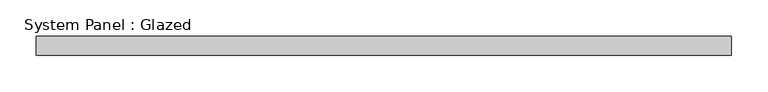
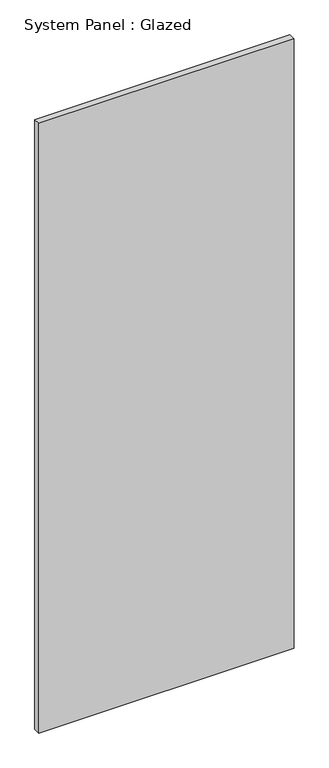
"""IFC4 building model written with IfcOpenShell, lengths in millimetres: plate geometry, System Panel : Glazed."""

from ifc_helpers import new_model, si_unit, origin, origin_with_axes, place, context, project, spatial, polyline, outline, extrude, source, transform, mapped, element, save


def system_panel_glazed_ce09be71(model_context):
    return source(origin(), model_context, "Body", "SweptSolid", [
        extrude(outline(polyline([(476.25, 19.05), (-476.25, 19.05), (-476.25, 44.45), (476.25, 44.45), (476.25, 19.05)])), origin_with_axes(), (0.0, 0.0, 1.0), 2402.4963211),
    ])


if __name__ == "__main__":
    model = new_model("IFC4")
    model_context = context("Model", 3, world=origin())
    ifc_project = project(units=[si_unit("LENGTHUNIT", "METRE", prefix="MILLI")], contexts=[model_context])
    site = spatial("IfcSite", under=ifc_project)
    building = spatial("IfcBuilding", under=site)
    placement = place(None, origin())
    system_panel_glazed_shape = system_panel_glazed_ce09be71(model_context)
    element("IfcPlate", 1, ObjectType="System Panel : Glazed", at=placement, inside=building, context=model_context, shape_type="MappedRepresentation", body=[
        mapped(system_panel_glazed_shape, transform((0.0, 0.0, 0.0), x_axis=(1.0, 0.0, 0.0), y_axis=(0.0, 1.0, 0.0), z_axis=(0.0, 0.0, 1.0))),
    ])
    save(model, "model.ifc")

# Revit data of these elements
# Type "System Panel : Glazed"
#   Construction Type Id = "GSP4R"
#   Analytic Construction = "1/8 in Pilkington single glazing"
#   Visual Light Transmittance = 0.9
#   Solar Heat Gain Coefficient = 0.86
#   Heat Transfer Coefficient (U) = 1.18115 BTU/(h·ft²·°F)
#   Define Thermal Properties by = 1
# Element 1 (IfcPlate, "System Panel : Glazed")
#   Materials on its faces: "Glass"
# Materials
#   "Glass": class "Glass", colour RGB 0 128 192, transparency 0.75, Description = "Soda Lime Glass", Cost = 0
